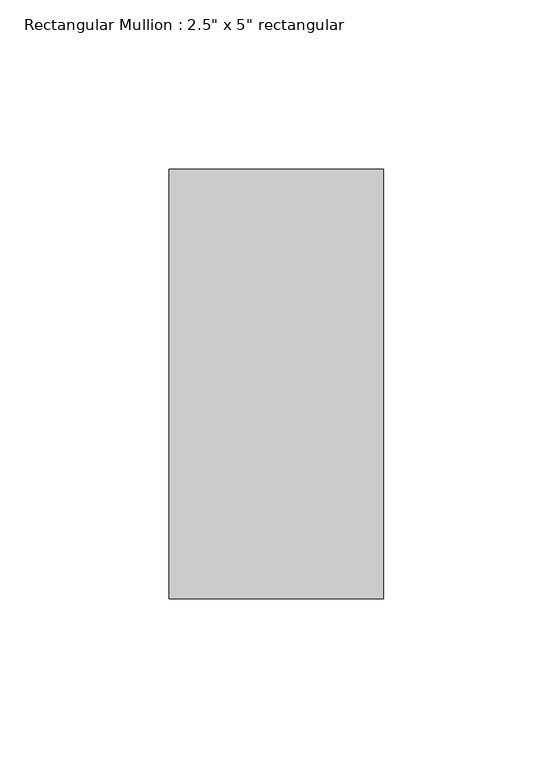
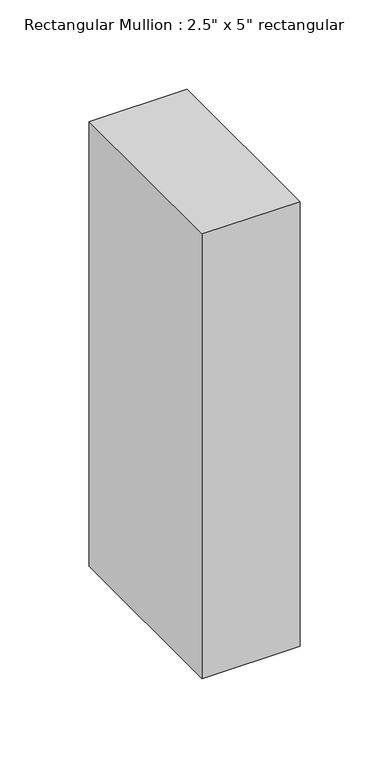
"""IFC4 building model written with IfcOpenShell, lengths in millimetres: member geometry."""

from ifc_helpers import new_model, si_unit, frame, origin, place, context, project, spatial, polyline, outline, extrude, source, transform, mapped, element, save


def member_3c3dc66a(model_context):
    return source(origin(), model_context, "Body", "SweptSolid", [
        extrude(outline(polyline([(0.0, 63.5), (0.0, -63.5), (-63.5, -63.5), (-63.5, 63.5), (0.0, 63.5)])), frame((0.0, 0.0, -304.8), z_axis=(0.0, 0.0, 1.0), x_axis=(1.0, 0.0, 0.0)), (0.0, 0.0, 1.0), 304.8),
    ])


if __name__ == "__main__":
    model = new_model("IFC4")
    model_context = context("Model", 3, world=origin())
    ifc_project = project(units=[si_unit("LENGTHUNIT", "METRE", prefix="MILLI")], contexts=[model_context])
    site = spatial("IfcSite", under=ifc_project)
    building = spatial("IfcBuilding", under=site)
    placement = place(None, origin())
    member_shape = member_3c3dc66a(model_context)
    element("IfcMember", 1, ObjectType="Rectangular Mullion : 2.5\" x 5\" rectangular", at=placement, inside=building, context=model_context, shape_type="MappedRepresentation", body=[
        mapped(member_shape, transform((0.0, 0.0, 0.0), x_axis=(1.0, 0.0, 0.0), y_axis=(0.0, 1.0, 0.0), z_axis=(0.0, 0.0, 1.0))),
    ])
    save(model, "model.ifc")

# Revit data of these elements
# Type "Rectangular Mullion : 2.5\" x 5\" rectangular"
#   built-in parameter 1007304 = 0.416667 (stored number, unit not read)
#   built-in parameter 1007301 = 0.104167 (stored number, unit not read)
#   built-in parameter 1007300 = 0.104167 (stored number, unit not read)
# Element 1 (IfcMember, "Rectangular Mullion : 2.5\" x 5\" rectangular")
#   Materials on its faces: "Aluminum"
# Materials
#   "Aluminum": class "Metal", colour RGB 247 247 247, transparency 0, Description = "Aluminum 6061", Cost = 0
